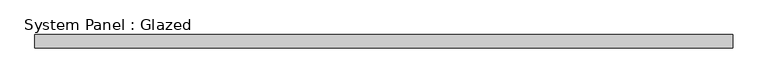
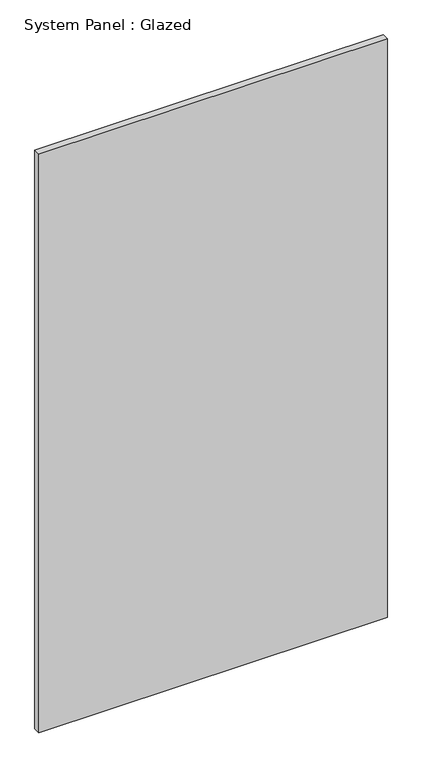
"""IFC4 building model written with IfcOpenShell, lengths in millimetres: plate geometry, System Panel : Glazed."""

from ifc_helpers import new_model, si_unit, origin, origin_with_axes, place, context, project, spatial, polyline, outline, extrude, source, transform, mapped, element, save


def system_panel_glazed_532211e4(model_context):
    return source(origin(), model_context, "Body", "SweptSolid", [
        extrude(outline(polyline([(667.8083334, 19.05), (-667.8083334, 19.05), (-667.8083334, 44.45), (667.8083334, 44.45), (667.8083334, 19.05)])), origin_with_axes(), (0.0, 0.0, 1.0), 2343.15),
    ])


if __name__ == "__main__":
    model = new_model("IFC4")
    model_context = context("Model", 3, world=origin())
    ifc_project = project(units=[si_unit("LENGTHUNIT", "METRE", prefix="MILLI")], contexts=[model_context])
    site = spatial("IfcSite", under=ifc_project)
    building = spatial("IfcBuilding", under=site)
    placement = place(None, origin())
    system_panel_glazed_shape = system_panel_glazed_532211e4(model_context)
    element("IfcPlate", 1, ObjectType="System Panel : Glazed", at=placement, inside=building, context=model_context, shape_type="MappedRepresentation", body=[
        mapped(system_panel_glazed_shape, transform((0.0, 0.0, 0.0), x_axis=(1.0, 0.0, 0.0), y_axis=(0.0, 1.0, 0.0), z_axis=(0.0, 0.0, 1.0))),
    ])
    save(model, "model.ifc")

# Revit data of these elements
# Type "System Panel : Glazed"
#   Construction Type Id = "GSP4R"
#   Analytic Construction = "1/8 in Pilkington single glazing"
#   Visual Light Transmittance = 0.9
#   Solar Heat Gain Coefficient = 0.86
#   Heat Transfer Coefficient (U) = 1.18115 BTU/(h·ft²·°F)
#   Define Thermal Properties by = 1
# Element 1 (IfcPlate, "System Panel : Glazed")
#   Materials on its faces: "Glass"
# Materials
#   "Glass": class "Glass", colour RGB 0 128 192, transparency 0.75, Description = "Soda Lime Glass", Cost = 0
